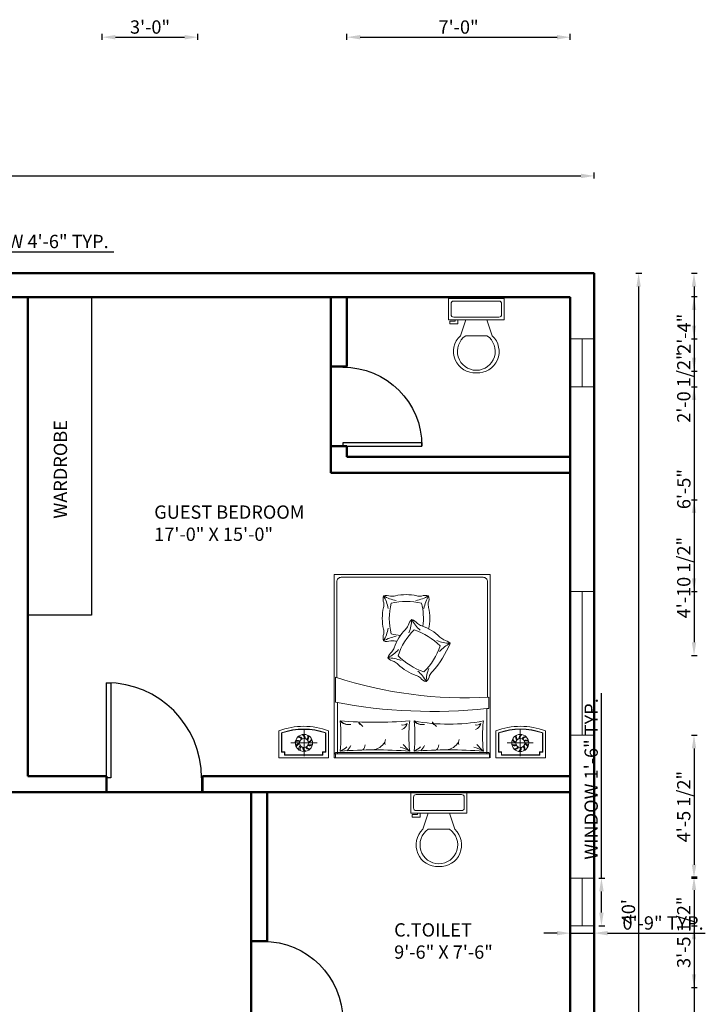
# Model space of a CAD drawing. Units: inches. Extents: x -46 to 764, y -530 to 112.
# Tile 5 of 5: x 507 to 764, y -262 to 108. Entities that reach past the tile are written whole.
import ezdxf

# ---------------------------------------------------------------- set-up
doc = ezdxf.new("R2010")
doc.units = ezdxf.units.IN
for name, color, linetype, lineweight in [('A-ANNO-DIMS', 2, 'Continuous', 18), ('A-AREA-IDEN', 7, 'Continuous', 18), ('A-DOOR', 3, 'Continuous', 25), ('A-FLOR-CASE', 32, 'Continuous', 25), ('A-FLOR-FIXT', 8, 'Continuous', 18), ('A-GLAZ', 4, 'Continuous', 18), ('A-WALL', 7, 'Continuous', 50), ('furn', 28, 'Continuous', 18), ('txt', 167, 'Continuous', 18)]:
    doc.layers.add(name, color=color, linetype=linetype, lineweight=lineweight)
doc.styles.get("Standard").update_dxf_attribs({"font": 'arial.ttf'})
doc.dimstyles.new('ISO-25', dxfattribs={"dimtxt": 5, "dimasz": 5, "dimexe": 1.25, "dimexo": 0.625, "dimtad": 1, "dimlunit": 3, "dimtxsty": 'Standard', "dimcen": 2.5, "dimadec": 0, "dimazin": 0, "dimtfac": 1, "dimtmove": 0, "dimatfit": 3, "dimfxl": 1, "dimfxlon": 1, "dimarcsym": 0})

# ---------------------------------------------------------------- blocks, each defined once
blk = doc.blocks.new('*U2')
for p, q in [((0, 0), (0, -6)), ((40, 0), (40, -6))]:
    blk.add_line(p, q)
blk.add_lwpolyline([(0, 0), (0, 40), (1.75, 40), (1.75, 0)], close=True)
blk.add_arc((0, 0), 40, 0, 90)
blk = doc.blocks.new('*U4')
for p, q in [((9.5, -6), (9.5, -2)), ((-10, -8.5), (-8, -8.5)), ((-10, -9.5), (-10, -8.5)), ((-7, -9.5), (-10, -9.5)), ((-8, -8.5), (-8, -8)), ((-7, -8), (-7, -9.5)), ((-4, -8), (-6, -14)), ((4, -8), (6, -14)), ((4, -14), (-4, -14))]:
    blk.add_line(p, q)
blk.add_lwpolyline([(10.5, -8), (10.5, 0), (-10.5, 0), (-10.5, -8)], close=True)
for points in [[(-9.5, -2), (-9.5, -6)], [(8.5, -1), (-8.5, -1)], [(-8.5, -7), (8.5, -7)]]:
    blk.add_lwpolyline(points)
for centre, radius, start, end in [((-8.625, -1.875), 0.8839, 81.8699, 188.1301), ((8.625, -1.875), 0.8839, 351.8699, 98.1301), ((-8.625, -6.125), 0.8839, 171.869898, 278.1301), ((8.625, -6.125), 0.8839, 261.8699, 8.1301), ((-0.4772, -19.9188), 8.0953, 133.01722, 273.38), ((0.0374, -19.8731), 7.127, 124.50543, 269.7), ((-0.0373, -19.8731), 7.127, 270.3, 55.4946), ((0.4773, -19.9188), 8.0953, 266.62, 46.9828)]:
    blk.add_arc(centre, radius, start, end)
blk = doc.blocks.new('*D10')
at = {"layer": 'A-ANNO-DIMS', "color": 0, "lineweight": -2, "transparency": 16777216}
for p, q in [((2.62, 48.57), (2.62, 50.82)), ((7.62, 49.57), (717.62, 49.57)), ((722.62, 48.57), (722.62, 50.82))]:
    blk.add_line(p, q, dxfattribs=at)
at = {"layer": 'A-ANNO-DIMS', "color": 0, "transparency": 16777216}
for points in [[(7.62, 50.4), (7.62, 48.73), (2.62, 49.57)], [(717.62, 50.4), (717.62, 48.73), (722.62, 49.57)]]:
    blk.add_solid(points, dxfattribs=at)
at = {"layer": 'Defpoints', "color": 0, "transparency": 16777216}
for p in [(722.62, 49.57), (2.62, 12.97), (722.62, 12.97)]:
    blk.add_point(p, dxfattribs=at)
at = {"layer": 'A-ANNO-DIMS', "color": 0, "transparency": 16777216, "insert": (362.62, 52.74), "char_height": 5, "attachment_point": 5}
blk.add_mtext("60'", dxfattribs=at)
blk = doc.blocks.new('*D11')
at = {"layer": 'A-ANNO-DIMS', "color": 0, "lineweight": -2, "transparency": 16777216}
for p, q in [((738.29, 12.97), (740.54, 12.97)), ((739.29, 7.97), (739.29, -462.03)), ((738.29, -467.03), (740.54, -467.03))]:
    blk.add_line(p, q, dxfattribs=at)
at = {"layer": 'A-ANNO-DIMS', "color": 0, "transparency": 16777216}
for points in [[(738.46, 7.97), (740.13, 7.97), (739.29, 12.97)], [(738.46, -462.03), (740.13, -462.03), (739.29, -467.03)]]:
    blk.add_solid(points, dxfattribs=at)
at = {"layer": 'Defpoints', "color": 0, "transparency": 16777216}
for p in [(722.62, 12.97), (722.62, -467.03), (739.29, -467.03)]:
    blk.add_point(p, dxfattribs=at)
at = {"layer": 'A-ANNO-DIMS', "color": 0, "transparency": 16777216, "insert": (736.12, -227.03), "char_height": 5, "attachment_point": 5, "rotation": 90}
blk.add_mtext("40'", dxfattribs=at)
blk = doc.blocks.new('BED-DOUBLE')
for p, q in [((1.34, 1.59), (1.34, 20.76)), ((57.43, 1.59), (57.43, 18.55)), ((57.72, 2.1), (1.02, 2.1))]:
    blk.add_line(p, q)
for points in [[(58.74, 0), (58.74, 68.93), (0, 68.93), (0, 0)], [(0.55, 0), (0.55, 1.59), (58.4, 1.59), (58.4, 0), (0, 0)]]:
    blk.add_lwpolyline(points)
for points in [[(57.72, 22.84), (57.72, 66.21, 0.414214), (56.03, 67.91), (2.72, 67.91, 0.414214), (1.02, 66.21), (1.02, 30.17)], [(18.6, 60.97, 0.159461), (18.72, 58.3, -0.076283), (18.6, 56.51, 0.115075), (18.6, 48.45, -0.076283), (18.72, 46.67, 0.159461), (18.6, 43.99)], [(20.35, 56.21, 0.091296), (18.6, 60.97, 0.091296), (23.37, 59.23)], [(30.8, 59.23, 0.091296), (35.58, 60.97, 0.091296), (33.82, 56.21, 0.091296)], [(32.9, 58.2, 0.111006), (21.48, 58.19, 0.119549), (21.48, 46.63, 0.033212), (24.99, 46.09)], [(29.21, 52.07, 0.159461), (27.9, 49.74, -0.076283), (26.85, 48.29, 0.115075), (22.59, 41.45, -0.076283), (21.75, 39.87, 0.159461), (20.23, 37.66)], [(28.18, 47.1, 0.091296), (29.21, 52.07, 0.091296), (32.34, 48.07)], [(23.37, 45.73, 0.091296), (18.6, 43.99, 0.091296), (20.35, 48.76, 0.091296)], [(39.88, 42.16, 0.111006), (30.18, 48.19, 0.119549), (24.07, 38.38, 0.107813), (33.74, 32.32)], [(25.2, 36.61, 0.091296), (20.23, 37.66, 0.091296), (24.24, 40.78, 0.091296)], [(33.79, 32.33, 0.121865), (39.88, 42.16, 0.121865)], [(38.65, 44.14, 0.091296), (43.62, 43.09, 0.091296), (39.61, 39.98, 0.091296)], [(35.68, 33.66, 0.091296), (34.64, 28.68, 0.091296), (31.51, 32.68, 0.091296)]]:
    blk.add_lwpolyline(points, format="xyb")
for points in [[(58.23, 18.55), (57.43, 18.55, -0.072944), (0.55, 20.92), (0.55, 30.34, 0.092568), (58.23, 22.87)], [(28.45, 13.91, 0.058596), (28.45, 2.57, 0.036648), (2.28, 2.57, 0.052163), (2.28, 13.91, 0.036967)], [(56.14, 13.91, 0.058596), (56.14, 2.57, 0.036889), (30.14, 2.57, 0.052163), (30.14, 13.91, 0.093111)]]:
    blk.add_lwpolyline(points, format="xyb", close=True)
for centre, radius, start, end in [((19.65, 56.16), 4.92, 70.7023, 102.284), ((21.76, 66.68), 5.9, 265.2252, 282.6741), ((27.14, 43.67), 17.74, 77.0576, 103.3153), ((32.37, 66.72), 5.9, 257.6988, 275.1477), ((34.43, 56.82), 4.3, 74.5791, 110.8198), ((31.43, 59.81), 4.3, 339.3666, 15.6073), ((9.55, 52.37), 24.07, 353.1956, 14.0284), ((41.33, 57.79), 5.9, 175.0387, 192.4877), ((18.3, 52.48), 17.74, 346.8711, 13.1289), ((27.56, 47.43), 4.92, 38.7754, 70.3571), ((34.92, 55.25), 5.9, 233.2983, 250.7472), ((27.31, 32.87), 17.74, 45.1307, 71.3884), ((43.94, 49.66), 5.9, 225.7718, 243.2208), ((19.87, 47.76), 3.97, 251.3996, 291.5774), ((21.86, 38.19), 5.9, 77.6988, 95.1477), ((27.09, 61.25), 17.74, 257.0576, 258.7033), ((9.2, 57.16), 37.18, 318.3818, 337.7644), ((40.46, 40.18), 4.3, 42.6522, 78.8929), ((23.3, 40.19), 3.97, 219.4726, 259.6505), ((19.93, 31.02), 5.9, 45.7718, 63.2208), ((36.56, 47.81), 17.74, 225.1307, 251.3884), ((28.95, 25.44), 5.9, 53.2983, 70.7472), ((35.78, 32.68), 4.15, 217.2937, 254.0973), ((31.74, 31.86), 4.3, 312.4658, 348.7065), ((41.21, 28.34), 5.9, 135.5854, 153.0343), ((4.9, 15.54), 2.94, 213.6349, 270.8456), ((5.76, 17.16), 4.64, 224.406, 276.8342), ((10.31, 13.43), 0.952, 173.7543, 257.2187), ((20.8, 21.81), 14.18, 216.2085, 225.0849), ((25.94, 14.96), 2.58, 256.4823, 308.5563), ((23.98, 14.17), 3.77, 294.2916, 340.9896), ((33.45, 17.16), 4.64, 224.406, 276.8342), ((32.59, 15.54), 2.94, 213.6349, 270.8456), ((38, 13.43), 0.952, 173.7543, 257.2187), ((48.49, 21.81), 14.18, 216.2085, 225.0849), ((53.63, 14.96), 2.58, 256.4823, 308.5563), ((51.67, 14.17), 3.77, 294.2916, 340.9896), ((-1.12, 10.34), 8.56, 294.6457, 314.1585), ((1.84, 6.34), 4.75, 310.5354, 340.3558), ((7.42, 5.72), 4.41, 321.8174, 349.8987), ((13.79, 9.29), 6.29, 276.6849, 328.3182), ((21.96, 5.79), 2.82, 155.8927, 196.1192), ((22.41, -6.92), 11.24, 57.5379, 77.5233), ((36.96, 13.18), 13.6, 216.4935, 231.2792), ((26.57, 10.34), 8.56, 294.6457, 314.1585), ((29.53, 6.34), 4.75, 310.5354, 340.3558), ((35.11, 5.72), 4.41, 321.8174, 349.8987), ((41.48, 9.29), 6.29, 276.6849, 328.3182), ((49.65, 5.79), 2.82, 155.8927, 196.1192), ((50.1, -6.92), 11.24, 57.5379, 77.5233), ((64.65, 13.18), 13.6, 216.4935, 231.2792), ((1.02, 1.08), 1.02, 90, 180), ((57.72, 1.08), 1.02, 0, 90)]:
    blk.add_arc(centre, radius, start, end)
blk = doc.blocks.new('NIGHTSTAND-L')
for p, q in [((9.43, 10.52), (9.43, 0.73)), ((4.54, 5.63), (14.33, 5.63))]:
    blk.add_line(p, q)
blk.add_lwpolyline([(0, 10.19), (0, 0), (18.68, 0), (18.68, 10.19, 0.181818)], format="xyb", close=True)
for points in [[(17.66, 2.14), (17.66, 9.48, 0.167087), (1.02, 9.48), (1.02, 2.14)], [(17.55, 2.14), (17.55, 9.4, 0.165559), (1.12, 9.4), (1.12, 2.14)]]:
    blk.add_lwpolyline(points, format="xyb")
for points in [[(2.24, 1.02), (2.24, 2.24), (1.02, 2.24)], [(2.14, 1.02), (2.14, 2.14), (1.02, 2.14)], [(2.14, 1.12), (16.54, 1.12)], [(2.14, 1.02), (16.54, 1.02)], [(16.43, 1.02), (16.43, 2.24), (17.66, 2.24)], [(16.54, 1.02), (16.54, 2.14), (17.66, 2.14)]]:
    blk.add_lwpolyline(points)
for radius in [3.2, 1.73]:
    blk.add_circle((9.43, 5.63), radius)
for centre, radius, start, end in [((7.17, 6.28), 1.57, 31.462, 91.6998), ((7.07, 6.1), 2.05, 33.5103, 79.83), ((7.98, 7.48), 1.57, 355.462, 55.6998), ((7.8, 7.4), 2.05, 357.5103, 43.83), ((9.35, 7.98), 1.57, 319.462, 19.6998), ((9.15, 8.02), 2.05, 321.5103, 7.83), ((6.99, 4.73), 1.57, 67.462, 127.6998), ((7.01, 4.53), 2.05, 69.5103, 115.83), ((8.02, 3.43), 2.05, 105.5103, 151.83), ((7.89, 3.59), 1.57, 103.462, 163.6998), ((9.48, 3.14), 2.05, 141.5103, 187.83), ((9.52, 3.28), 1.57, 139.462, 199.6998), ((11.07, 3.86), 2.05, 177.5103, 223.83), ((10.88, 3.77), 1.57, 175.462, 235.6998), ((11.8, 5.16), 2.05, 213.5103, 259.83), ((11.7, 4.98), 1.57, 211.462, 271.6998), ((11.63, 6.64), 2.05, 249.5103, 295.83), ((11.64, 6.43), 1.57, 247.462, 307.6998), ((10.75, 7.58), 1.57, 283.462, 343.6998), ((10.61, 7.73), 2.05, 285.5103, 331.83)]:
    blk.add_arc(centre, radius, start, end)
blk = doc.blocks.new('NIGHTSTAND-R')
for p, q in [((9.24, 10.52), (9.24, 0.73)), ((14.14, 5.62), (4.35, 5.62))]:
    blk.add_line(p, q)
blk.add_lwpolyline([(18.68, 10.19), (18.68, 0), (0, 0), (0, 10.19, -0.181818)], format="xyb", close=True)
for points in [[(1.02, 2.14), (1.02, 9.48, -0.167087), (17.66, 9.48), (17.66, 2.14)], [(1.12, 2.14), (1.12, 9.4, -0.165559), (17.56, 9.4), (17.56, 2.14)]]:
    blk.add_lwpolyline(points, format="xyb")
for points in [[(2.24, 1.02), (2.24, 2.24), (1.02, 2.24)], [(2.14, 1.02), (2.14, 2.14), (1.02, 2.14)], [(16.54, 1.12), (2.14, 1.12)], [(16.54, 1.02), (2.14, 1.02)], [(16.43, 1.02), (16.43, 2.24), (17.66, 2.24)], [(16.54, 1.02), (16.54, 2.14), (17.66, 2.14)]]:
    blk.add_lwpolyline(points)
for radius in [3.2, 1.73]:
    blk.add_circle((9.24, 5.62), radius)
for centre, radius, start, end in [((9.52, 8.02), 2.05, 172.17, 218.4897), ((9.32, 7.97), 1.57, 160.3002, 220.538), ((10.88, 7.4), 2.05, 136.17, 182.4897), ((10.69, 7.48), 1.57, 124.3002, 184.538), ((11.61, 6.09), 2.05, 100.17, 146.4897), ((11.5, 6.27), 1.57, 88.3002, 148.538), ((7.03, 6.43), 1.57, 232.3002, 292.538), ((7.05, 6.63), 2.05, 244.17, 290.4897), ((8.06, 7.73), 2.05, 208.17, 254.4897), ((7.93, 7.57), 1.57, 196.3002, 256.538), ((6.98, 4.98), 1.57, 268.3002, 328.538), ((6.88, 5.15), 2.05, 280.17, 326.4897), ((7.79, 3.77), 1.57, 304.3002, 4.538), ((7.6, 3.85), 2.05, 316.17, 2.4897), ((9.16, 3.27), 1.57, 340.3002, 40.538), ((8.96, 3.23), 2.05, 352.17, 38.4897), ((11.43, 4.61), 2.05, 64.17, 110.4897), ((11.45, 4.82), 1.57, 52.3002, 112.538), ((10.56, 3.67), 1.57, 16.3002, 76.538), ((10.42, 3.52), 2.05, 28.17, 74.4897)]:
    blk.add_arc(centre, radius, start, end)
blk = doc.blocks.new('WIN-54IN')
blk.add_line((4.5, 54), (4.5, 0))
blk.add_lwpolyline([(0, 54), (9, 54), (9, 0), (0, 0)], close=True)
blk = doc.blocks.new('WIN-18IN')
blk.add_line((4.5, 18), (4.5, 0))
blk.add_lwpolyline([(0, 18), (9, 18), (9, 0), (0, 0)], close=True)
blk = doc.blocks.new('*D19')
at = {"layer": 'A-ANNO-DIMS', "color": 0, "lineweight": -2, "transparency": 16777216}
for p, q in [((418.45, 20.07), (418.45, 22.32)), ((472.45, 20.07), (472.45, 22.32)), ((423.45, 21.07), (467.45, 21.07)), ((472.45, 21.07), (541.97, 21.07))]:
    blk.add_line(p, q, dxfattribs=at)
at = {"layer": 'A-ANNO-DIMS', "color": 0, "transparency": 16777216}
for points in [[(423.45, 21.9), (423.45, 20.24), (418.45, 21.07)], [(467.45, 21.9), (467.45, 20.24), (472.45, 21.07)]]:
    blk.add_solid(points, dxfattribs=at)
at = {"layer": 'Defpoints', "color": 0, "transparency": 16777216}
for p in [(472.45, 21.07), (418.45, 12.97), (472.45, 12.97)]:
    blk.add_point(p, dxfattribs=at)
at = {"layer": 'A-ANNO-DIMS', "color": 0, "transparency": 16777216, "insert": (509.71, 24.28), "char_height": 5, "attachment_point": 5}
blk.add_mtext('WINDOW 4\'-6" TYP.', dxfattribs=at)
blk = doc.blocks.new('*D23')
at = {"layer": 'A-ANNO-DIMS', "color": 0, "lineweight": -2, "transparency": 16777216}
for p, q in [((725.32, -214.39), (725.32, -144.87)), ((724.32, -214.39), (726.57, -214.39)), ((725.32, -227.39), (725.32, -219.39)), ((724.32, -232.39), (726.57, -232.39))]:
    blk.add_line(p, q, dxfattribs=at)
at = {"layer": 'A-ANNO-DIMS', "color": 0, "transparency": 16777216}
for points in [[(724.49, -219.39), (726.16, -219.39), (725.32, -214.39)], [(724.49, -227.39), (726.16, -227.39), (725.32, -232.39)]]:
    blk.add_solid(points, dxfattribs=at)
at = {"layer": 'Defpoints', "color": 0, "transparency": 16777216}
for p in [(722.62, -214.39), (725.32, -214.39), (722.62, -232.39)]:
    blk.add_point(p, dxfattribs=at)
at = {"layer": 'A-ANNO-DIMS', "color": 0, "transparency": 16777216, "insert": (722.11, -177.13), "char_height": 5, "attachment_point": 5, "rotation": 90}
blk.add_mtext('WINDOW 1\'-6" TYP.', dxfattribs=at)
blk = doc.blocks.new('*D24')
at = {"layer": 'A-ANNO-DIMS', "color": 0, "lineweight": -2, "transparency": 16777216}
for p, q in [((708.62, -235.09), (703.62, -235.09)), ((713.62, -234.09), (713.62, -236.34)), ((713.62, -235.09), (722.62, -235.09)), ((722.62, -234.09), (722.62, -236.34)), ((727.62, -235.09), (764.35, -235.09))]:
    blk.add_line(p, q, dxfattribs=at)
at = {"layer": 'A-ANNO-DIMS', "color": 0, "transparency": 16777216}
for points in [[(708.62, -234.26), (708.62, -235.92), (713.62, -235.09)], [(727.62, -234.26), (727.62, -235.92), (722.62, -235.09)]]:
    blk.add_solid(points, dxfattribs=at)
at = {"layer": 'Defpoints', "color": 0, "transparency": 16777216}
for p in [(713.62, -232.39), (722.62, -232.39), (722.62, -235.09)]:
    blk.add_point(p, dxfattribs=at)
at = {"layer": 'A-ANNO-DIMS', "color": 0, "transparency": 16777216, "insert": (748.49, -231.91), "char_height": 5, "attachment_point": 5}
blk.add_mtext('0\'-9" TYP.', dxfattribs=at)
blk = doc.blocks.new('*D42')
at = {"layer": 'A-ANNO-DIMS', "color": 0, "lineweight": -2, "transparency": 16777216}
for p, q in [((759.12, -72.15), (761.37, -72.15)), ((760.12, -77.15), (760.12, -125.72)), ((759.12, -130.72), (761.37, -130.72))]:
    blk.add_line(p, q, dxfattribs=at)
at = {"layer": 'A-ANNO-DIMS', "color": 0, "transparency": 16777216}
for points in [[(759.29, -77.15), (760.96, -77.15), (760.12, -72.15)], [(759.29, -125.72), (760.96, -125.72), (760.12, -130.72)]]:
    blk.add_solid(points, dxfattribs=at)
at = {"layer": 'Defpoints', "color": 0, "transparency": 16777216}
for p in [(448.74, -72.15), (448.74, -130.72), (760.12, -130.72)]:
    blk.add_point(p, dxfattribs=at)
at = {"layer": 'A-ANNO-DIMS', "color": 0, "transparency": 16777216, "insert": (756.91, -101.44), "char_height": 5, "attachment_point": 5, "rotation": 90}
blk.add_mtext('4\'-10 1/2"', dxfattribs=at)
blk = doc.blocks.new('*D47')
at = {"layer": 'A-ANNO-DIMS', "color": 0, "lineweight": -2, "transparency": 16777216}
for p, q in [((629.62, 100.72), (629.62, 102.97)), ((634.62, 101.72), (708.62, 101.72)), ((713.62, 100.72), (713.62, 102.97))]:
    blk.add_line(p, q, dxfattribs=at)
at = {"layer": 'A-ANNO-DIMS', "color": 0, "transparency": 16777216}
for points in [[(634.62, 102.55), (634.62, 100.88), (629.62, 101.72)], [(708.62, 102.55), (708.62, 100.88), (713.62, 101.72)]]:
    blk.add_solid(points, dxfattribs=at)
at = {"layer": 'Defpoints', "color": 0, "transparency": 16777216}
for p in [(713.62, 101.72), (629.62, -56.03), (713.62, -56.03)]:
    blk.add_point(p, dxfattribs=at)
at = {"layer": 'A-ANNO-DIMS', "color": 0, "transparency": 16777216, "insert": (671.62, 104.89), "char_height": 5, "attachment_point": 5}
blk.add_mtext('7\'-0"', dxfattribs=at)
blk = doc.blocks.new('*D48')
at = {"layer": 'A-ANNO-DIMS', "color": 0, "lineweight": -2, "transparency": 16777216}
for p, q in [((-33.88, 3.97), (-36.13, 3.97)), ((-34.88, -1.03), (-34.88, -51.03)), ((-33.88, -56.03), (-36.13, -56.03))]:
    blk.add_line(p, q, dxfattribs=at)
at = {"layer": 'A-ANNO-DIMS', "color": 0, "transparency": 16777216}
for points in [[(-35.71, -1.03), (-34.04, -1.03), (-34.88, 3.97)], [(-35.71, -51.03), (-34.04, -51.03), (-34.88, -56.03)]]:
    blk.add_solid(points, dxfattribs=at)
at = {"layer": 'Defpoints', "color": 0, "transparency": 16777216}
for p in [(713.62, 3.97), (-34.88, -56.03), (713.62, -56.03)]:
    blk.add_point(p, dxfattribs=at)
at = {"layer": 'A-ANNO-DIMS', "color": 0, "transparency": 16777216, "insert": (-38.05, -26.03), "char_height": 5, "attachment_point": 5, "rotation": 90}
blk.add_mtext('5\'-0"', dxfattribs=at)
blk = doc.blocks.new('*D58')
at = {"layer": 'A-ANNO-DIMS', "color": 0, "lineweight": -2, "transparency": 16777216}
for p, q in [((759.12, 12.97), (761.37, 12.97)), ((760.12, 7.97), (760.12, -6.67)), ((759.12, -11.67), (761.37, -11.67)), ((760.12, -11.67), (760.12, -42.94))]:
    blk.add_line(p, q, dxfattribs=at)
at = {"layer": 'A-ANNO-DIMS', "color": 0, "transparency": 16777216}
for points in [[(759.29, 7.97), (760.96, 7.97), (760.12, 12.97)], [(759.29, -6.67), (760.96, -6.67), (760.12, -11.67)]]:
    blk.add_solid(points, dxfattribs=at)
at = {"layer": 'Defpoints', "color": 0, "transparency": 16777216}
for p in [(722.62, 12.97), (722.62, -11.67), (760.12, -11.67)]:
    blk.add_point(p, dxfattribs=at)
at = {"layer": 'A-ANNO-DIMS', "color": 0, "transparency": 16777216, "insert": (756.91, -29.81), "char_height": 5, "attachment_point": 5, "rotation": 90}
blk.add_mtext('2\'-0 1/2"', dxfattribs=at)
blk = doc.blocks.new('*D59')
at = {"layer": 'A-ANNO-DIMS', "color": 0, "lineweight": -2, "transparency": 16777216}
for p, q in [((759.12, -29.67), (761.37, -29.67)), ((760.12, -34.67), (760.12, -101.65)), ((759.12, -106.65), (761.37, -106.65))]:
    blk.add_line(p, q, dxfattribs=at)
at = {"layer": 'A-ANNO-DIMS', "color": 0, "transparency": 16777216}
for points in [[(759.29, -34.67), (760.96, -34.67), (760.12, -29.67)], [(759.29, -101.65), (760.96, -101.65), (760.12, -106.65)]]:
    blk.add_solid(points, dxfattribs=at)
at = {"layer": 'Defpoints', "color": 0, "transparency": 16777216}
for p in [(722.62, -29.67), (722.62, -106.65), (760.12, -106.65)]:
    blk.add_point(p, dxfattribs=at)
at = {"layer": 'A-ANNO-DIMS', "color": 0, "transparency": 16777216, "insert": (756.95, -68.16), "char_height": 5, "attachment_point": 5, "rotation": 90}
blk.add_mtext('6\'-5"', dxfattribs=at)
blk = doc.blocks.new('*D60')
at = {"layer": 'A-ANNO-DIMS', "color": 0, "lineweight": -2, "transparency": 16777216}
for p, q in [((759.12, -160.65), (761.37, -160.65)), ((760.12, -165.65), (760.12, -209.39)), ((759.12, -214.39), (761.37, -214.39))]:
    blk.add_line(p, q, dxfattribs=at)
at = {"layer": 'A-ANNO-DIMS', "color": 0, "transparency": 16777216}
for points in [[(759.29, -165.65), (760.96, -165.65), (760.12, -160.65)], [(759.29, -209.39), (760.96, -209.39), (760.12, -214.39)]]:
    blk.add_solid(points, dxfattribs=at)
at = {"layer": 'Defpoints', "color": 0, "transparency": 16777216}
for p in [(722.62, -160.65), (722.62, -214.39), (760.12, -214.39)]:
    blk.add_point(p, dxfattribs=at)
at = {"layer": 'A-ANNO-DIMS', "color": 0, "transparency": 16777216, "insert": (756.91, -187.52), "char_height": 5, "attachment_point": 5, "rotation": 90}
blk.add_mtext('4\'-5 1/2"', dxfattribs=at)
blk = doc.blocks.new('*D61')
at = {"layer": 'A-ANNO-DIMS', "color": 0, "lineweight": -2, "transparency": 16777216}
for p, q in [((759.12, -232.39), (761.37, -232.39)), ((760.12, -237.39), (760.12, -358.93)), ((759.12, -363.93), (761.37, -363.93))]:
    blk.add_line(p, q, dxfattribs=at)
at = {"layer": 'A-ANNO-DIMS', "color": 0, "transparency": 16777216}
for points in [[(759.29, -237.39), (760.96, -237.39), (760.12, -232.39)], [(759.29, -358.93), (760.96, -358.93), (760.12, -363.93)]]:
    blk.add_solid(points, dxfattribs=at)
at = {"layer": 'Defpoints', "color": 0, "transparency": 16777216}
for p in [(722.62, -232.39), (722.62, -363.93), (760.12, -363.93)]:
    blk.add_point(p, dxfattribs=at)
at = {"layer": 'A-ANNO-DIMS', "color": 0, "transparency": 16777216, "insert": (756.91, -298.16), "char_height": 5, "attachment_point": 5, "rotation": 90}
blk.add_mtext('10\'-11 1/2"', dxfattribs=at)
blk = doc.blocks.new('*D77')
at = {"layer": 'A-ANNO-DIMS', "color": 0, "lineweight": -2, "transparency": 16777216}
for p, q in [((537.62, 100.72), (537.62, 102.97)), ((542.62, 101.72), (568.62, 101.72)), ((573.62, 100.72), (573.62, 102.97))]:
    blk.add_line(p, q, dxfattribs=at)
at = {"layer": 'A-ANNO-DIMS', "color": 0, "transparency": 16777216}
for points in [[(542.62, 102.55), (542.62, 100.88), (537.62, 101.72)], [(568.62, 102.55), (568.62, 100.88), (573.62, 101.72)]]:
    blk.add_solid(points, dxfattribs=at)
at = {"layer": 'Defpoints', "color": 0, "transparency": 16777216}
for p in [(573.62, 101.72), (537.62, -272.03), (573.62, -272.03)]:
    blk.add_point(p, dxfattribs=at)
at = {"layer": 'A-ANNO-DIMS', "color": 0, "transparency": 16777216, "insert": (555.62, 104.9), "char_height": 5, "attachment_point": 5}
blk.add_mtext('3\'-0"', dxfattribs=at)
blk = doc.blocks.new('*D81')
at = {"layer": 'A-ANNO-DIMS', "color": 0, "lineweight": -2, "transparency": 16777216}
for p, q in [((759.12, -213.92), (761.37, -213.92)), ((760.12, -218.92), (760.12, -250.58)), ((759.12, -255.58), (761.37, -255.58))]:
    blk.add_line(p, q, dxfattribs=at)
at = {"layer": 'A-ANNO-DIMS', "color": 0, "transparency": 16777216}
for points in [[(759.29, -218.92), (760.96, -218.92), (760.12, -213.92)], [(759.29, -250.58), (760.96, -250.58), (760.12, -255.58)]]:
    blk.add_solid(points, dxfattribs=at)
at = {"layer": 'Defpoints', "color": 0, "transparency": 16777216}
for p in [(139.44, -213.92), (139.44, -255.58), (760.12, -255.58)]:
    blk.add_point(p, dxfattribs=at)
at = {"layer": 'A-ANNO-DIMS', "color": 0, "transparency": 16777216, "insert": (756.91, -234.75), "char_height": 5, "attachment_point": 5, "rotation": 90}
blk.add_mtext('3\'-5 1/2"', dxfattribs=at)
blk = doc.blocks.new('*D83')
at = {"layer": 'A-ANNO-DIMS', "color": 0, "lineweight": -2, "transparency": 16777216}
for p, q in [((759.12, 4.22), (761.37, 4.22)), ((760.12, -0.78), (760.12, -18.78)), ((759.12, -23.78), (761.37, -23.78))]:
    blk.add_line(p, q, dxfattribs=at)
at = {"layer": 'A-ANNO-DIMS', "color": 0, "transparency": 16777216}
for points in [[(759.29, -0.78), (760.96, -0.78), (760.12, 4.22)], [(759.29, -18.78), (760.96, -18.78), (760.12, -23.78)]]:
    blk.add_solid(points, dxfattribs=at)
at = {"layer": 'Defpoints', "color": 0, "transparency": 16777216}
for p in [(54.53, 4.22), (44.03, -23.78), (760.12, -23.78)]:
    blk.add_point(p, dxfattribs=at)
at = {"layer": 'A-ANNO-DIMS', "color": 0, "transparency": 16777216, "insert": (756.99, -9.78), "char_height": 5, "attachment_point": 5, "rotation": 90}
blk.add_mtext('2\'-4"', dxfattribs=at)

msp = doc.modelspace()

# ---------------------------------------------------------------- linework, layer by layer
at = {"layer": 'A-FLOR-CASE'}
for p, q in [((533.624, 3.97), (533.624, -115.509)), ((533.624, -115.509), (509.624, -115.509))]:
    msp.add_line(p, q, dxfattribs=at)
at = {"layer": 'A-WALL'}
for p, q in [((2.624, 12.97), (722.624, 12.97)), ((722.624, 12.97), (722.624, -467.03)), ((337.047, 3.97), (713.624, 3.97)), ((509.624, 3.97), (509.624, -176.03)), ((623.624, -62.03), (623.624, 3.97)), ((629.624, -22.03), (629.624, 3.97)), ((713.624, 3.97), (713.624, -458.03)), ((629.624, -22.03), (623.624, -22.03)), ((629.624, -52.03), (623.624, -52.03)), ((629.624, -56.03), (629.624, -52.03)), ((713.624, -56.03), (629.624, -56.03)), ((629.624, -62.03), (623.624, -62.03)), ((713.624, -62.03), (629.624, -62.03)), ((509.624, -176.03), (539.294, -176.03)), ((539.294, -182.03), (539.294, -176.03)), ((575.294, -182.03), (575.294, -176.03)), ((575.294, -176.03), (713.624, -176.03)), ((509.624, -182.03), (503.624, -182.03)), ((509.624, -182.03), (713.624, -182.03)), ((593.624, -182.03), (593.624, -272.03)), ((599.624, -182.03), (599.624, -238.107)), ((599.624, -238.107), (593.624, -238.107))]:
    msp.add_line(p, q, dxfattribs=at)

# ---------------------------------------------------------------- block references
at = {"layer": 'A-DOOR', "rotation": 270}
for p, xscale, yscale, zscale in [((628.085, -52.024), -0.7435414179882275, 0.7435414179882275, 0.7435414179882275), ((598.119, -268.107), -0.7492007242236776, 0.7492007242236776, 0.7492007242236776)]:
    msp.add_blockref('*U2', p, dxfattribs=dict(at, xscale=xscale, yscale=yscale, zscale=zscale))
at = {"layer": 'A-DOOR', "xscale": 0.8921564434138556, "yscale": 0.8921564434138556, "zscale": 0.8921564434138556}
msp.add_blockref('*U2', (539.294, -176.677), dxfattribs=at)
at = {"layer": 'A-FLOR-FIXT'}
for p in [(678.287, 3.503), (664.202, -182.03)]:
    msp.add_blockref('*U4', p, dxfattribs=at)
at = {"layer": 'A-GLAZ'}
for name, p in [('WIN-18IN', (713.624, -29.668)), ('WIN-54IN', (713.624, -160.654)), ('WIN-18IN', (713.624, -232.39))]:
    msp.add_blockref(name, p, dxfattribs=at)
at = {"layer": 'furn'}
for name, p in [('BED-DOUBLE', (624.789, -169.232)), ('NIGHTSTAND-L', (604.076, -169.231)), ('NIGHTSTAND-R', (685.569, -169.228))]:
    msp.add_blockref(name, p, dxfattribs=at)

# ---------------------------------------------------------------- texts
at = {"layer": 'A-AREA-IDEN', "char_height": 5, "attachment_point": 1}
for s, width, insert in [('GUEST BEDROOM\\P17\'-0" X 15\'-0"', 67.58637, (557.202, -74.301)), ('C.TOILET\\P9\'-6" X 7\'-6"', 52.48842, (647.395, -231.374))]:
    msp.add_mtext_dynamic_manual_height_columns(s, width=width, gutter_width=12.5, heights=[0], dxfattribs=dict(at, insert=insert))
at = {"layer": 'txt', "insert": (519.439, -79.273), "char_height": 5, "attachment_point": 1, "rotation": 90}
msp.add_mtext_dynamic_manual_height_columns('WARDROBE', width=154.75533, gutter_width=12.5, heights=[0], dxfattribs=at)

# ---------------------------------------------------------------- dimensions: what is measured, and where the dimension line sits
at = {"layer": 'A-ANNO-DIMS'}
for base, p1, p2, override, picture, middle in [((573.624, 101.716), (537.624, -272.03), (573.624, -272.03), {"dimdec": 1, "dimlfac": 1, "dimrnd": 0, "dimzin": 1, "dimdsep": 46, "dimlunit": 4, "dimfrac": 2}, '*D77', (555.624, 104.896)), ((713.624, 101.716), (629.624, -56.03), (713.624, -56.03), {"dimdec": 1, "dimlfac": 1, "dimrnd": 0, "dimzin": 1, "dimdsep": 46, "dimlunit": 4, "dimfrac": 2}, '*D47', (671.624, 104.894)), ((722.624, 49.565), (2.624, 12.97), (722.624, 12.97), {"dimclrd": 0, "dimclre": 0, "dimclrt": 0}, '*D10', (362.624, 52.743))]:
    dim = msp.add_linear_dim(base=base, p1=p1, p2=p2, dimstyle='ISO-25', override=override, dxfattribs=at)
    dim.commit()
    dim.dimension.update_dxf_attribs({"geometry": picture, "text_midpoint": middle})
for base, p1, p2, text, picture, middle in [((472.448, 21.07), (418.448, 12.97), (472.448, 12.97), 'WINDOW <> TYP.', '*D19', (509.709, 24.282)), ((722.624, -235.09), (713.624, -232.39), (722.624, -232.39), '<> TYP.', '*D24', (748.488, -231.912))]:
    dim = msp.add_linear_dim(base=base, p1=p1, p2=p2, text=text, dimstyle='ISO-25', override={"dimdec": 1, "dimlfac": 1, "dimrnd": 0, "dimzin": 1, "dimdsep": 46, "dimlunit": 4, "dimfrac": 2}, dxfattribs=at)
    dim.commit()
    dim.dimension.update_dxf_attribs({"geometry": picture, "text_midpoint": middle})
for base, p1, p2, override, picture, middle in [((739.294, -467.03), (722.624, 12.97), (722.624, -467.03), {"dimclrd": 0, "dimclre": 0, "dimclrt": 0}, '*D11', (736.116, -227.03)), ((760.124, -11.667), (722.624, 12.97), (722.624, -11.667), {"dimdec": 1, "dimlfac": 1, "dimrnd": 0, "dimzin": 1, "dimdsep": 46, "dimlunit": 4, "dimfrac": 2}, '*D58', (756.914, -29.806)), ((-34.876, -56.03), (713.624, 3.97), (713.624, -56.03), {"dimdec": 1, "dimlfac": 1, "dimrnd": 0, "dimzin": 1, "dimdsep": 46, "dimlunit": 4, "dimfrac": 2}, '*D48', (-38.054, -26.03)), ((760.124, -23.784), (54.533, 4.216), (44.033, -23.784), {"dimdec": 1, "dimlfac": 1, "dimrnd": 0, "dimzin": 1, "dimdsep": 46, "dimlunit": 4, "dimfrac": 2}, '*D83', (756.989, -9.784)), ((760.124, -106.654), (722.624, -29.667), (722.624, -106.654), {"dimdec": 1, "dimlfac": 1, "dimrnd": 0, "dimzin": 1, "dimdsep": 46, "dimlunit": 4, "dimfrac": 2}, '*D59', (756.946, -68.161)), ((760.124, -130.719), (448.744, -72.153), (448.744, -130.719), {"dimdec": 1, "dimlfac": 1, "dimrnd": 0, "dimzin": 1, "dimdsep": 46, "dimlunit": 4, "dimfrac": 2}, '*D42', (756.914, -101.436)), ((760.124, -214.39), (722.624, -160.654), (722.624, -214.39), {"dimdec": 1, "dimlfac": 1, "dimrnd": 0, "dimzin": 1, "dimdsep": 46, "dimlunit": 4, "dimfrac": 2}, '*D60', (756.914, -187.522)), ((760.124, -255.575), (139.438, -213.915), (139.438, -255.575), {"dimdec": 1, "dimlfac": 1, "dimrnd": 0, "dimzin": 1, "dimdsep": 46, "dimlunit": 4, "dimfrac": 2}, '*D81', (756.912, -234.745)), ((760.124, -363.925), (722.624, -232.39), (722.624, -363.925), {"dimdec": 1, "dimlfac": 1, "dimrnd": 0, "dimzin": 1, "dimdsep": 46, "dimlunit": 4, "dimfrac": 2}, '*D61', (756.914, -298.157))]:
    dim = msp.add_linear_dim(base=base, p1=p1, p2=p2, angle=90, dimstyle='ISO-25', override=override, dxfattribs=at)
    dim.commit()
    dim.dimension.update_dxf_attribs({"geometry": picture, "text_midpoint": middle})
dim = msp.add_linear_dim(base=(725.324, -214.39), p1=(722.624, -232.39), p2=(722.624, -214.39), angle=90, text='WINDOW <> TYP.', dimstyle='ISO-25', override={"dimdec": 1, "dimlfac": 1, "dimrnd": 0, "dimzin": 1, "dimdsep": 46, "dimlunit": 4, "dimfrac": 2}, dxfattribs=at)
dim.commit()
dim.dimension.update_dxf_attribs({"geometry": '*D23', "text_midpoint": (722.112, -177.129)})

doc.saveas('drawing.dxf')
